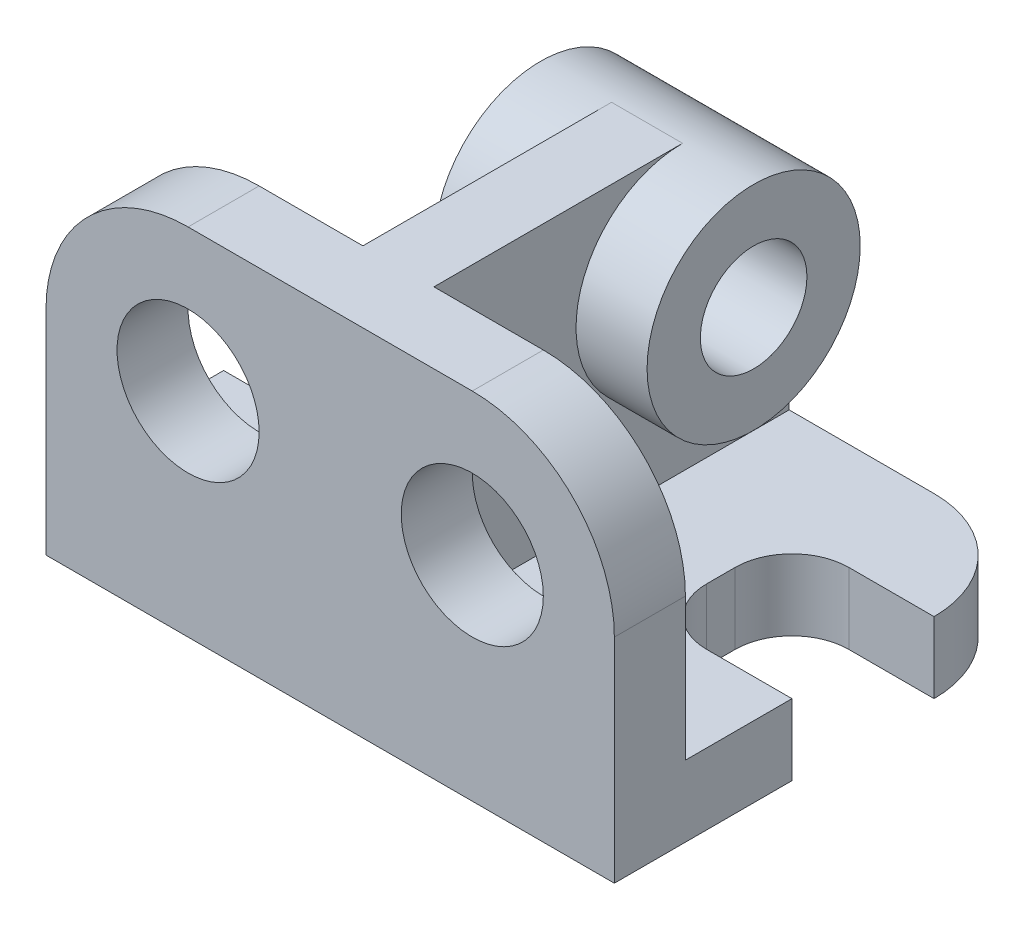
ISO-10303-21;
HEADER;
FILE_DESCRIPTION(('STEP AP214'),'2;1');
FILE_NAME('part.step','',(''),(''),'','','');
FILE_SCHEMA(('AUTOMOTIVE_DESIGN { 1 0 10303 214 1 1 1 1 }'));
ENDSEC;
DATA;
#1=APPLICATION_CONTEXT('core data for automotive mechanical design processes');
#2=APPLICATION_PROTOCOL_DEFINITION('international standard','automotive_design',2000,#1);
#3=PRODUCT_CONTEXT('',#1,'mechanical');
#4=PRODUCT('Part','Part','',(#3));
#5=PRODUCT_RELATED_PRODUCT_CATEGORY('part','',(#4));
#6=PRODUCT_DEFINITION_FORMATION('','',#4);
#7=PRODUCT_DEFINITION_CONTEXT('part definition',#1,'design');
#8=PRODUCT_DEFINITION('design','',#6,#7);
#9=PRODUCT_DEFINITION_SHAPE('','',#8);
#10=(LENGTH_UNIT() NAMED_UNIT(*) SI_UNIT(.MILLI.,.METRE.));
#11=(NAMED_UNIT(*) PLANE_ANGLE_UNIT() SI_UNIT($,.RADIAN.));
#12=(NAMED_UNIT(*) SI_UNIT($,.STERADIAN.) SOLID_ANGLE_UNIT());
#13=UNCERTAINTY_MEASURE_WITH_UNIT(LENGTH_MEASURE(1.E-05),#10,'distance_accuracy_value','');
#14=(GEOMETRIC_REPRESENTATION_CONTEXT(3) GLOBAL_UNCERTAINTY_ASSIGNED_CONTEXT((#13)) GLOBAL_UNIT_ASSIGNED_CONTEXT((#10,
#11,#12)) REPRESENTATION_CONTEXT('',''));
#15=CARTESIAN_POINT('',(0.,0.,0.));
#16=DIRECTION('',(0.,0.,1.));
#17=DIRECTION('',(1.,0.,0.));
#18=AXIS2_PLACEMENT_3D('',#15,#16,#17);
#19=CARTESIAN_POINT('',(-2.49999999999999,1.,-3.));
#20=DIRECTION('',(0.,0.,1.));
#21=DIRECTION('',(1.,0.,0.));
#22=AXIS2_PLACEMENT_3D('',#19,#20,#21);
#23=PLANE('',#22);
#24=DIRECTION('',(1.,0.,0.));
#25=VECTOR('',#24,1.);
#26=CARTESIAN_POINT('',(-2.53950180731732,3.5,-3.));
#27=LINE('',#26,#25);
#28=CARTESIAN_POINT('',(-0.539501807317321,3.5,-3.));
#29=VERTEX_POINT('',#28);
#30=CARTESIAN_POINT('',(0.460498192682678,3.5,-3.));
#31=VERTEX_POINT('',#30);
#32=EDGE_CURVE('E202',#29,#31,#27,.T.);
#33=ORIENTED_EDGE('',*,*,#32,.T.);
#34=DIRECTION('',(0.,-1.,0.));
#35=VECTOR('',#34,1.);
#36=CARTESIAN_POINT('',(0.460498192682678,1.,-3.));
#37=LINE('',#36,#35);
#38=CARTESIAN_POINT('',(0.460498192682678,1.,-3.));
#39=VERTEX_POINT('',#38);
#40=EDGE_CURVE('E208',#31,#39,#37,.T.);
#41=ORIENTED_EDGE('',*,*,#40,.T.);
#42=DIRECTION('',(-1.,0.,0.));
#43=VECTOR('',#42,1.);
#44=CARTESIAN_POINT('',(-2.49999999999999,1.,-3.));
#45=LINE('',#44,#43);
#46=CARTESIAN_POINT('',(2.49999999999999,1.,-3.));
#47=VERTEX_POINT('',#46);
#48=EDGE_CURVE('E307',#47,#39,#45,.T.);
#49=ORIENTED_EDGE('',*,*,#48,.F.);
#50=DIRECTION('',(0.,-1.,0.));
#51=VECTOR('',#50,1.);
#52=CARTESIAN_POINT('',(2.49999999999999,1.,-3.));
#53=LINE('',#52,#51);
#54=CARTESIAN_POINT('',(2.49999999999999,0.,-3.));
#55=VERTEX_POINT('',#54);
#56=EDGE_CURVE('E375',#47,#55,#53,.T.);
#57=ORIENTED_EDGE('',*,*,#56,.T.);
#58=DIRECTION('',(-1.,0.,0.));
#59=VECTOR('',#58,1.);
#60=CARTESIAN_POINT('',(-2.49999999999999,0.,-3.));
#61=LINE('',#60,#59);
#62=CARTESIAN_POINT('',(-2.49999999999999,0.,-3.));
#63=VERTEX_POINT('',#62);
#64=EDGE_CURVE('E338',#55,#63,#61,.T.);
#65=ORIENTED_EDGE('',*,*,#64,.T.);
#66=DIRECTION('',(0.,-1.,0.));
#67=VECTOR('',#66,1.);
#68=CARTESIAN_POINT('',(-2.49999999999999,1.,-3.));
#69=LINE('',#68,#67);
#70=CARTESIAN_POINT('',(-2.49999999999999,1.,-3.));
#71=VERTEX_POINT('',#70);
#72=EDGE_CURVE('E369',#71,#63,#69,.T.);
#73=ORIENTED_EDGE('',*,*,#72,.F.);
#74=CARTESIAN_POINT('',(-0.539501807317322,1.,-3.));
#75=VERTEX_POINT('',#74);
#76=EDGE_CURVE('E308',#75,#71,#45,.T.);
#77=ORIENTED_EDGE('',*,*,#76,.F.);
#78=DIRECTION('',(0.,1.,0.));
#79=VECTOR('',#78,1.);
#80=CARTESIAN_POINT('',(-0.539501807317321,5.,-3.));
#81=LINE('',#80,#79);
#82=EDGE_CURVE('E211',#75,#29,#81,.T.);
#83=ORIENTED_EDGE('',*,*,#82,.T.);
#84=EDGE_LOOP('',(#33,#41,#49,#57,#65,#73,#77,#83));
#85=FACE_BOUND('',#84,.T.);
#86=ADVANCED_FACE('F39',(#85),#23,.F.);
#87=CARTESIAN_POINT('',(-1.99999999999999,5.,2.));
#88=DIRECTION('',(0.,1.,0.));
#89=DIRECTION('',(0.,0.,1.));
#90=AXIS2_PLACEMENT_3D('',#87,#88,#89);
#91=PLANE('',#90);
#92=DIRECTION('',(0.,0.,1.));
#93=VECTOR('',#92,1.);
#94=CARTESIAN_POINT('',(0.460498192682678,5.,-3.));
#95=LINE('',#94,#93);
#96=CARTESIAN_POINT('',(0.460498192682678,5.,-1.5));
#97=VERTEX_POINT('',#96);
#98=CARTESIAN_POINT('',(0.460498192682678,5.,2.));
#99=VERTEX_POINT('',#98);
#100=EDGE_CURVE('E233',#97,#99,#95,.T.);
#101=ORIENTED_EDGE('',*,*,#100,.F.);
#102=DIRECTION('',(1.,0.,0.));
#103=VECTOR('',#102,1.);
#104=CARTESIAN_POINT('',(-2.53950180731732,5.,-1.5));
#105=LINE('',#104,#103);
#106=CARTESIAN_POINT('',(-0.539501807317321,5.,-1.5));
#107=VERTEX_POINT('',#106);
#108=EDGE_CURVE('E53',#107,#97,#105,.T.);
#109=ORIENTED_EDGE('',*,*,#108,.F.);
#110=DIRECTION('',(0.,0.,1.));
#111=VECTOR('',#110,1.);
#112=CARTESIAN_POINT('',(-0.539501807317321,5.,-3.));
#113=LINE('',#112,#111);
#114=CARTESIAN_POINT('',(-0.539501807317322,5.,2.));
#115=VERTEX_POINT('',#114);
#116=EDGE_CURVE('E58',#107,#115,#113,.T.);
#117=ORIENTED_EDGE('',*,*,#116,.T.);
#118=DIRECTION('',(-1.,0.,0.));
#119=VECTOR('',#118,1.);
#120=CARTESIAN_POINT('',(-1.99999999999999,5.,2.));
#121=LINE('',#120,#119);
#122=CARTESIAN_POINT('',(-1.99999999999999,5.,2.));
#123=VERTEX_POINT('',#122);
#124=EDGE_CURVE('E265',#115,#123,#121,.T.);
#125=ORIENTED_EDGE('',*,*,#124,.T.);
#126=DIRECTION('',(0.,0.,1.));
#127=VECTOR('',#126,1.);
#128=CARTESIAN_POINT('',(-1.99999999999999,5.,2.));
#129=LINE('',#128,#127);
#130=CARTESIAN_POINT('',(-1.99999999999999,5.,3.));
#131=VERTEX_POINT('',#130);
#132=EDGE_CURVE('E273',#123,#131,#129,.T.);
#133=ORIENTED_EDGE('',*,*,#132,.T.);
#134=DIRECTION('',(-1.,0.,0.));
#135=VECTOR('',#134,1.);
#136=CARTESIAN_POINT('',(-1.99999999999999,5.,3.));
#137=LINE('',#136,#135);
#138=CARTESIAN_POINT('',(1.99999999999999,5.,3.));
#139=VERTEX_POINT('',#138);
#140=EDGE_CURVE('E255',#139,#131,#137,.T.);
#141=ORIENTED_EDGE('',*,*,#140,.F.);
#142=DIRECTION('',(0.,0.,1.));
#143=VECTOR('',#142,1.);
#144=CARTESIAN_POINT('',(1.99999999999999,5.,2.));
#145=LINE('',#144,#143);
#146=CARTESIAN_POINT('',(1.99999999999999,5.,2.));
#147=VERTEX_POINT('',#146);
#148=EDGE_CURVE('E280',#147,#139,#145,.T.);
#149=ORIENTED_EDGE('',*,*,#148,.F.);
#150=EDGE_CURVE('E263',#147,#99,#121,.T.);
#151=ORIENTED_EDGE('',*,*,#150,.T.);
#152=EDGE_LOOP('',(#101,#109,#117,#125,#133,#141,#149,#151));
#153=FACE_BOUND('',#152,.T.);
#154=ADVANCED_FACE('F453',(#153),#91,.T.);
#155=CARTESIAN_POINT('',(-0.539501807317321,5.,-3.));
#156=DIRECTION('',(1.,0.,0.));
#157=DIRECTION('',(0.,1.,0.));
#158=AXIS2_PLACEMENT_3D('',#155,#156,#157);
#159=PLANE('',#158);
#160=ORIENTED_EDGE('',*,*,#116,.F.);
#161=CARTESIAN_POINT('',(-0.539501807317322,3.5,-1.5));
#162=DIRECTION('',(1.,0.,0.));
#163=DIRECTION('',(0.,1.,0.));
#164=AXIS2_PLACEMENT_3D('',#161,#162,#163);
#165=CIRCLE('',#164,1.5);
#166=EDGE_CURVE('E231',#107,#29,#165,.T.);
#167=ORIENTED_EDGE('',*,*,#166,.T.);
#168=ORIENTED_EDGE('',*,*,#82,.F.);
#169=DIRECTION('',(0.,0.,1.));
#170=VECTOR('',#169,1.);
#171=CARTESIAN_POINT('',(-0.539501807317322,1.,-3.));
#172=LINE('',#171,#170);
#173=CARTESIAN_POINT('',(-0.539501807317322,1.,2.));
#174=VERTEX_POINT('',#173);
#175=EDGE_CURVE('E225',#75,#174,#172,.T.);
#176=ORIENTED_EDGE('',*,*,#175,.T.);
#177=DIRECTION('',(0.,1.,0.));
#178=VECTOR('',#177,1.);
#179=CARTESIAN_POINT('',(-0.539501807317321,5.,2.));
#180=LINE('',#179,#178);
#181=EDGE_CURVE('E228',#174,#115,#180,.T.);
#182=ORIENTED_EDGE('',*,*,#181,.T.);
#183=EDGE_LOOP('',(#160,#167,#168,#176,#182));
#184=FACE_BOUND('',#183,.T.);
#185=ADVANCED_FACE('F478',(#184),#159,.F.);
#186=CARTESIAN_POINT('',(-2.8,1.,-0.3));
#187=DIRECTION('',(0.,-1.,0.));
#188=DIRECTION('',(0.,0.,-1.));
#189=AXIS2_PLACEMENT_3D('',#186,#187,#188);
#190=PLANE('',#189);
#191=ORIENTED_EDGE('',*,*,#175,.F.);
#192=ORIENTED_EDGE('',*,*,#76,.T.);
#193=CARTESIAN_POINT('',(-2.5,1.,-1.5));
#194=DIRECTION('',(0.,1.,0.));
#195=DIRECTION('',(0.,0.,1.));
#196=AXIS2_PLACEMENT_3D('',#193,#194,#195);
#197=CIRCLE('',#196,1.5);
#198=CARTESIAN_POINT('',(-4.,1.,-1.49999999999999));
#199=VERTEX_POINT('',#198);
#200=EDGE_CURVE('E310',#71,#199,#197,.T.);
#201=ORIENTED_EDGE('',*,*,#200,.T.);
#202=DIRECTION('',(1.,0.,0.));
#203=VECTOR('',#202,1.);
#204=CARTESIAN_POINT('',(-4.,1.,-1.49999999999999));
#205=LINE('',#204,#203);
#206=CARTESIAN_POINT('',(-2.80000000000001,1.,-1.5));
#207=VERTEX_POINT('',#206);
#208=EDGE_CURVE('E313',#199,#207,#205,.T.);
#209=ORIENTED_EDGE('',*,*,#208,.T.);
#210=CARTESIAN_POINT('',(-2.8,1.,-0.699999999999996));
#211=DIRECTION('',(0.,-1.,0.));
#212=DIRECTION('',(0.,0.,1.));
#213=AXIS2_PLACEMENT_3D('',#210,#211,#212);
#214=CIRCLE('',#213,0.8);
#215=CARTESIAN_POINT('',(-2.,1.,-0.69999999999999));
#216=VERTEX_POINT('',#215);
#217=EDGE_CURVE('E311',#207,#216,#214,.T.);
#218=ORIENTED_EDGE('',*,*,#217,.T.);
#219=DIRECTION('',(0.,0.,1.));
#220=VECTOR('',#219,1.);
#221=CARTESIAN_POINT('',(-2.,1.,-0.69999999999999));
#222=LINE('',#221,#220);
#223=CARTESIAN_POINT('',(-2.,1.,-0.300000000000006));
#224=VERTEX_POINT('',#223);
#225=EDGE_CURVE('E312',#216,#224,#222,.T.);
#226=ORIENTED_EDGE('',*,*,#225,.T.);
#227=CARTESIAN_POINT('',(-2.8,1.,-0.3));
#228=DIRECTION('',(0.,-1.,0.));
#229=DIRECTION('',(0.,0.,-1.));
#230=AXIS2_PLACEMENT_3D('',#227,#228,#229);
#231=CIRCLE('',#230,0.8);
#232=CARTESIAN_POINT('',(-2.80000000000001,1.,0.5));
#233=VERTEX_POINT('',#232);
#234=EDGE_CURVE('E320',#224,#233,#231,.T.);
#235=ORIENTED_EDGE('',*,*,#234,.T.);
#236=DIRECTION('',(-1.,0.,0.));
#237=VECTOR('',#236,1.);
#238=CARTESIAN_POINT('',(-2.80000000000001,1.,0.5));
#239=LINE('',#238,#237);
#240=CARTESIAN_POINT('',(-4.,1.,0.5));
#241=VERTEX_POINT('',#240);
#242=EDGE_CURVE('E317',#233,#241,#239,.T.);
#243=ORIENTED_EDGE('',*,*,#242,.T.);
#244=DIRECTION('',(0.,0.,1.));
#245=VECTOR('',#244,1.);
#246=CARTESIAN_POINT('',(-4.,1.,3.));
#247=LINE('',#246,#245);
#248=CARTESIAN_POINT('',(-4.,1.,2.));
#249=VERTEX_POINT('',#248);
#250=EDGE_CURVE('E289',#241,#249,#247,.T.);
#251=ORIENTED_EDGE('',*,*,#250,.T.);
#252=DIRECTION('',(-1.,0.,0.));
#253=VECTOR('',#252,1.);
#254=CARTESIAN_POINT('',(-2.8,1.,2.));
#255=LINE('',#254,#253);
#256=EDGE_CURVE('E277',#174,#249,#255,.T.);
#257=ORIENTED_EDGE('',*,*,#256,.F.);
#258=EDGE_LOOP('',(#191,#192,#201,#209,#218,#226,#235,#243,#251,#257));
#259=FACE_BOUND('',#258,.T.);
#260=ADVANCED_FACE('F417',(#259),#190,.F.);
#261=DIRECTION('',(0.,0.,1.));
#262=VECTOR('',#261,1.);
#263=CARTESIAN_POINT('',(0.460498192682678,1.,-3.));
#264=LINE('',#263,#262);
#265=CARTESIAN_POINT('',(0.460498192682678,1.,2.));
#266=VERTEX_POINT('',#265);
#267=EDGE_CURVE('E219',#39,#266,#264,.T.);
#268=ORIENTED_EDGE('',*,*,#267,.T.);
#269=CARTESIAN_POINT('',(4.,1.,2.));
#270=VERTEX_POINT('',#269);
#271=EDGE_CURVE('E283',#270,#266,#255,.T.);
#272=ORIENTED_EDGE('',*,*,#271,.F.);
#273=DIRECTION('',(0.,0.,-1.));
#274=VECTOR('',#273,1.);
#275=CARTESIAN_POINT('',(4.,1.,3.));
#276=LINE('',#275,#274);
#277=CARTESIAN_POINT('',(4.,1.,0.5));
#278=VERTEX_POINT('',#277);
#279=EDGE_CURVE('E292',#270,#278,#276,.T.);
#280=ORIENTED_EDGE('',*,*,#279,.T.);
#281=DIRECTION('',(-1.,0.,0.));
#282=VECTOR('',#281,1.);
#283=CARTESIAN_POINT('',(2.80000000000001,1.,0.5));
#284=LINE('',#283,#282);
#285=CARTESIAN_POINT('',(2.80000000000001,1.,0.5));
#286=VERTEX_POINT('',#285);
#287=EDGE_CURVE('E294',#278,#286,#284,.T.);
#288=ORIENTED_EDGE('',*,*,#287,.T.);
#289=CARTESIAN_POINT('',(2.8,1.,-0.3));
#290=DIRECTION('',(0.,-1.,0.));
#291=DIRECTION('',(0.,0.,1.));
#292=AXIS2_PLACEMENT_3D('',#289,#290,#291);
#293=CIRCLE('',#292,0.8);
#294=CARTESIAN_POINT('',(2.,1.,-0.300000000000006));
#295=VERTEX_POINT('',#294);
#296=EDGE_CURVE('E296',#286,#295,#293,.T.);
#297=ORIENTED_EDGE('',*,*,#296,.T.);
#298=DIRECTION('',(0.,0.,-1.));
#299=VECTOR('',#298,1.);
#300=CARTESIAN_POINT('',(2.,1.,-0.69999999999999));
#301=LINE('',#300,#299);
#302=CARTESIAN_POINT('',(2.,1.,-0.69999999999999));
#303=VERTEX_POINT('',#302);
#304=EDGE_CURVE('E299',#295,#303,#301,.T.);
#305=ORIENTED_EDGE('',*,*,#304,.T.);
#306=CARTESIAN_POINT('',(2.8,1.,-0.699999999999996));
#307=DIRECTION('',(0.,-1.,0.));
#308=DIRECTION('',(0.,0.,-1.));
#309=AXIS2_PLACEMENT_3D('',#306,#307,#308);
#310=CIRCLE('',#309,0.8);
#311=CARTESIAN_POINT('',(2.8,1.,-1.5));
#312=VERTEX_POINT('',#311);
#313=EDGE_CURVE('E300',#303,#312,#310,.T.);
#314=ORIENTED_EDGE('',*,*,#313,.T.);
#315=DIRECTION('',(1.,0.,0.));
#316=VECTOR('',#315,1.);
#317=CARTESIAN_POINT('',(4.,1.,-1.49999999999999));
#318=LINE('',#317,#316);
#319=CARTESIAN_POINT('',(4.,1.,-1.49999999999999));
#320=VERTEX_POINT('',#319);
#321=EDGE_CURVE('E302',#312,#320,#318,.T.);
#322=ORIENTED_EDGE('',*,*,#321,.T.);
#323=CARTESIAN_POINT('',(2.5,1.,-1.5));
#324=DIRECTION('',(0.,1.,0.));
#325=DIRECTION('',(0.,0.,-1.));
#326=AXIS2_PLACEMENT_3D('',#323,#324,#325);
#327=CIRCLE('',#326,1.5);
#328=EDGE_CURVE('E303',#320,#47,#327,.T.);
#329=ORIENTED_EDGE('',*,*,#328,.T.);
#330=ORIENTED_EDGE('',*,*,#48,.T.);
#331=EDGE_LOOP('',(#268,#272,#280,#288,#297,#305,#314,#322,#329,#330));
#332=FACE_BOUND('',#331,.T.);
#333=ADVANCED_FACE('F442',(#332),#190,.F.);
#334=CARTESIAN_POINT('',(-2.,3.,2.));
#335=DIRECTION('',(0.,0.,1.));
#336=DIRECTION('',(1.,0.,0.));
#337=AXIS2_PLACEMENT_3D('',#334,#335,#336);
#338=PLANE('',#337);
#339=CARTESIAN_POINT('',(-2.,3.,2.));
#340=DIRECTION('',(0.,0.,1.));
#341=DIRECTION('',(1.,0.,0.));
#342=AXIS2_PLACEMENT_3D('',#339,#340,#341);
#343=CIRCLE('',#342,1.);
#344=CARTESIAN_POINT('',(-1.,3.,2.));
#345=VERTEX_POINT('',#344);
#346=EDGE_CURVE('E243',#345,#345,#343,.T.);
#347=ORIENTED_EDGE('',*,*,#346,.T.);
#348=EDGE_LOOP('',(#347));
#349=FACE_BOUND('',#348,.T.);
#350=ORIENTED_EDGE('',*,*,#181,.F.);
#351=ORIENTED_EDGE('',*,*,#256,.T.);
#352=DIRECTION('',(0.,-1.,0.));
#353=VECTOR('',#352,1.);
#354=CARTESIAN_POINT('',(-4.,0.,2.));
#355=LINE('',#354,#353);
#356=CARTESIAN_POINT('',(-4.,2.99999999999999,2.));
#357=VERTEX_POINT('',#356);
#358=EDGE_CURVE('E251',#357,#249,#355,.T.);
#359=ORIENTED_EDGE('',*,*,#358,.F.);
#360=CARTESIAN_POINT('',(-2.,3.,2.));
#361=DIRECTION('',(0.,0.,1.));
#362=DIRECTION('',(1.,0.,0.));
#363=AXIS2_PLACEMENT_3D('',#360,#361,#362);
#364=CIRCLE('',#363,2.);
#365=EDGE_CURVE('E250',#123,#357,#364,.T.);
#366=ORIENTED_EDGE('',*,*,#365,.F.);
#367=ORIENTED_EDGE('',*,*,#124,.F.);
#368=EDGE_LOOP('',(#350,#351,#359,#366,#367));
#369=FACE_BOUND('',#368,.T.);
#370=ADVANCED_FACE('F411',(#349,#369),#338,.F.);
#371=CARTESIAN_POINT('',(2.,3.,2.));
#372=DIRECTION('',(0.,0.,1.));
#373=DIRECTION('',(1.,0.,0.));
#374=AXIS2_PLACEMENT_3D('',#371,#372,#373);
#375=CIRCLE('',#374,1.);
#376=CARTESIAN_POINT('',(3.,3.,2.));
#377=VERTEX_POINT('',#376);
#378=EDGE_CURVE('E236',#377,#377,#375,.T.);
#379=ORIENTED_EDGE('',*,*,#378,.T.);
#380=EDGE_LOOP('',(#379));
#381=FACE_BOUND('',#380,.T.);
#382=DIRECTION('',(0.,-1.,0.));
#383=VECTOR('',#382,1.);
#384=CARTESIAN_POINT('',(0.460498192682678,1.,2.));
#385=LINE('',#384,#383);
#386=EDGE_CURVE('E223',#99,#266,#385,.T.);
#387=ORIENTED_EDGE('',*,*,#386,.F.);
#388=ORIENTED_EDGE('',*,*,#150,.F.);
#389=CARTESIAN_POINT('',(2.,3.,2.));
#390=DIRECTION('',(0.,0.,1.));
#391=DIRECTION('',(-1.,0.,0.));
#392=AXIS2_PLACEMENT_3D('',#389,#390,#391);
#393=CIRCLE('',#392,2.);
#394=CARTESIAN_POINT('',(4.,2.99999999999999,2.));
#395=VERTEX_POINT('',#394);
#396=EDGE_CURVE('E259',#395,#147,#393,.T.);
#397=ORIENTED_EDGE('',*,*,#396,.F.);
#398=DIRECTION('',(0.,1.,0.));
#399=VECTOR('',#398,1.);
#400=CARTESIAN_POINT('',(4.,0.,2.));
#401=LINE('',#400,#399);
#402=EDGE_CURVE('E260',#270,#395,#401,.T.);
#403=ORIENTED_EDGE('',*,*,#402,.F.);
#404=ORIENTED_EDGE('',*,*,#271,.T.);
#405=EDGE_LOOP('',(#387,#388,#397,#403,#404));
#406=FACE_BOUND('',#405,.T.);
#407=ADVANCED_FACE('F449',(#381,#406),#338,.F.);
#408=CARTESIAN_POINT('',(-4.,1.,3.));
#409=DIRECTION('',(1.,0.,0.));
#410=DIRECTION('',(0.,0.,-1.));
#411=AXIS2_PLACEMENT_3D('',#408,#409,#410);
#412=PLANE('',#411);
#413=DIRECTION('',(0.,-1.,0.));
#414=VECTOR('',#413,1.);
#415=CARTESIAN_POINT('',(-4.,1.,3.));
#416=LINE('',#415,#414);
#417=CARTESIAN_POINT('',(-4.,2.99999999999999,3.));
#418=VERTEX_POINT('',#417);
#419=CARTESIAN_POINT('',(-4.,0.,3.));
#420=VERTEX_POINT('',#419);
#421=EDGE_CURVE('E50',#418,#420,#416,.T.);
#422=ORIENTED_EDGE('',*,*,#421,.F.);
#423=DIRECTION('',(0.,0.,1.));
#424=VECTOR('',#423,1.);
#425=CARTESIAN_POINT('',(-4.,2.99999999999999,2.));
#426=LINE('',#425,#424);
#427=EDGE_CURVE('E266',#357,#418,#426,.T.);
#428=ORIENTED_EDGE('',*,*,#427,.F.);
#429=ORIENTED_EDGE('',*,*,#358,.T.);
#430=ORIENTED_EDGE('',*,*,#250,.F.);
#431=DIRECTION('',(0.,-1.,0.));
#432=VECTOR('',#431,1.);
#433=CARTESIAN_POINT('',(-4.,1.,0.5));
#434=LINE('',#433,#432);
#435=CARTESIAN_POINT('',(-4.,0.,0.5));
#436=VERTEX_POINT('',#435);
#437=EDGE_CURVE('E321',#241,#436,#434,.T.);
#438=ORIENTED_EDGE('',*,*,#437,.T.);
#439=DIRECTION('',(0.,0.,1.));
#440=VECTOR('',#439,1.);
#441=CARTESIAN_POINT('',(-4.,0.,3.));
#442=LINE('',#441,#440);
#443=EDGE_CURVE('E287',#436,#420,#442,.T.);
#444=ORIENTED_EDGE('',*,*,#443,.T.);
#445=EDGE_LOOP('',(#422,#428,#429,#430,#438,#444));
#446=FACE_BOUND('',#445,.T.);
#447=ADVANCED_FACE('F41',(#446),#412,.F.);
#448=CARTESIAN_POINT('',(-4.,1.,3.));
#449=DIRECTION('',(0.,0.,-1.));
#450=DIRECTION('',(-1.,0.,0.));
#451=AXIS2_PLACEMENT_3D('',#448,#449,#450);
#452=PLANE('',#451);
#453=DIRECTION('',(1.,0.,0.));
#454=VECTOR('',#453,1.);
#455=CARTESIAN_POINT('',(-4.,0.,3.));
#456=LINE('',#455,#454);
#457=CARTESIAN_POINT('',(4.,0.,3.));
#458=VERTEX_POINT('',#457);
#459=EDGE_CURVE('E323',#420,#458,#456,.T.);
#460=ORIENTED_EDGE('',*,*,#459,.T.);
#461=DIRECTION('',(0.,-1.,0.));
#462=VECTOR('',#461,1.);
#463=CARTESIAN_POINT('',(4.,1.,3.));
#464=LINE('',#463,#462);
#465=CARTESIAN_POINT('',(4.,2.99999999999999,3.));
#466=VERTEX_POINT('',#465);
#467=EDGE_CURVE('E394',#466,#458,#464,.T.);
#468=ORIENTED_EDGE('',*,*,#467,.F.);
#469=CARTESIAN_POINT('',(2.,3.,3.));
#470=DIRECTION('',(0.,0.,1.));
#471=DIRECTION('',(-1.,0.,0.));
#472=AXIS2_PLACEMENT_3D('',#469,#470,#471);
#473=CIRCLE('',#472,2.);
#474=EDGE_CURVE('E267',#466,#139,#473,.T.);
#475=ORIENTED_EDGE('',*,*,#474,.T.);
#476=ORIENTED_EDGE('',*,*,#140,.T.);
#477=CARTESIAN_POINT('',(-2.,3.,3.));
#478=DIRECTION('',(0.,0.,1.));
#479=DIRECTION('',(1.,0.,0.));
#480=AXIS2_PLACEMENT_3D('',#477,#478,#479);
#481=CIRCLE('',#480,2.);
#482=EDGE_CURVE('E247',#131,#418,#481,.T.);
#483=ORIENTED_EDGE('',*,*,#482,.T.);
#484=ORIENTED_EDGE('',*,*,#421,.T.);
#485=EDGE_LOOP('',(#460,#468,#475,#476,#483,#484));
#486=FACE_BOUND('',#485,.T.);
#487=CARTESIAN_POINT('',(-2.,3.,3.));
#488=DIRECTION('',(0.,0.,1.));
#489=DIRECTION('',(1.,0.,0.));
#490=AXIS2_PLACEMENT_3D('',#487,#488,#489);
#491=CIRCLE('',#490,1.);
#492=CARTESIAN_POINT('',(-1.,3.,3.));
#493=VERTEX_POINT('',#492);
#494=EDGE_CURVE('E241',#493,#493,#491,.T.);
#495=ORIENTED_EDGE('',*,*,#494,.F.);
#496=EDGE_LOOP('',(#495));
#497=FACE_BOUND('',#496,.T.);
#498=CARTESIAN_POINT('',(2.,3.,3.));
#499=DIRECTION('',(0.,0.,1.));
#500=DIRECTION('',(1.,0.,0.));
#501=AXIS2_PLACEMENT_3D('',#498,#499,#500);
#502=CIRCLE('',#501,1.);
#503=CARTESIAN_POINT('',(3.,3.,3.));
#504=VERTEX_POINT('',#503);
#505=EDGE_CURVE('E240',#504,#504,#502,.T.);
#506=ORIENTED_EDGE('',*,*,#505,.F.);
#507=EDGE_LOOP('',(#506));
#508=FACE_BOUND('',#507,.T.);
#509=ADVANCED_FACE('F397',(#486,#497,#508),#452,.F.);
#510=CARTESIAN_POINT('',(4.,1.,3.));
#511=DIRECTION('',(-1.,0.,0.));
#512=DIRECTION('',(0.,0.,1.));
#513=AXIS2_PLACEMENT_3D('',#510,#511,#512);
#514=PLANE('',#513);
#515=DIRECTION('',(0.,0.,-1.));
#516=VECTOR('',#515,1.);
#517=CARTESIAN_POINT('',(4.,0.,3.));
#518=LINE('',#517,#516);
#519=CARTESIAN_POINT('',(4.,0.,0.5));
#520=VERTEX_POINT('',#519);
#521=EDGE_CURVE('E324',#458,#520,#518,.T.);
#522=ORIENTED_EDGE('',*,*,#521,.T.);
#523=DIRECTION('',(0.,-1.,0.));
#524=VECTOR('',#523,1.);
#525=CARTESIAN_POINT('',(4.,1.,0.5));
#526=LINE('',#525,#524);
#527=EDGE_CURVE('E388',#278,#520,#526,.T.);
#528=ORIENTED_EDGE('',*,*,#527,.F.);
#529=ORIENTED_EDGE('',*,*,#279,.F.);
#530=ORIENTED_EDGE('',*,*,#402,.T.);
#531=DIRECTION('',(0.,0.,1.));
#532=VECTOR('',#531,1.);
#533=CARTESIAN_POINT('',(4.,2.99999999999999,2.));
#534=LINE('',#533,#532);
#535=EDGE_CURVE('E276',#395,#466,#534,.T.);
#536=ORIENTED_EDGE('',*,*,#535,.T.);
#537=ORIENTED_EDGE('',*,*,#467,.T.);
#538=EDGE_LOOP('',(#522,#528,#529,#530,#536,#537));
#539=FACE_BOUND('',#538,.T.);
#540=ADVANCED_FACE('F433',(#539),#514,.F.);
#541=CARTESIAN_POINT('',(2.80000000000001,1.,0.5));
#542=DIRECTION('',(0.,0.,1.));
#543=DIRECTION('',(1.,0.,0.));
#544=AXIS2_PLACEMENT_3D('',#541,#542,#543);
#545=PLANE('',#544);
#546=DIRECTION('',(-1.,0.,0.));
#547=VECTOR('',#546,1.);
#548=CARTESIAN_POINT('',(2.80000000000001,0.,0.5));
#549=LINE('',#548,#547);
#550=CARTESIAN_POINT('',(2.80000000000001,0.,0.5));
#551=VERTEX_POINT('',#550);
#552=EDGE_CURVE('E330',#520,#551,#549,.T.);
#553=ORIENTED_EDGE('',*,*,#552,.T.);
#554=DIRECTION('',(0.,-1.,0.));
#555=VECTOR('',#554,1.);
#556=CARTESIAN_POINT('',(2.80000000000001,1.,0.5));
#557=LINE('',#556,#555);
#558=EDGE_CURVE('E390',#286,#551,#557,.T.);
#559=ORIENTED_EDGE('',*,*,#558,.F.);
#560=ORIENTED_EDGE('',*,*,#287,.F.);
#561=ORIENTED_EDGE('',*,*,#527,.T.);
#562=EDGE_LOOP('',(#553,#559,#560,#561));
#563=FACE_BOUND('',#562,.T.);
#564=ADVANCED_FACE('F440',(#563),#545,.F.);
#565=CARTESIAN_POINT('',(2.8,1.,-0.3));
#566=DIRECTION('',(0.,-1.,0.));
#567=DIRECTION('',(0.,0.,-1.));
#568=AXIS2_PLACEMENT_3D('',#565,#566,#567);
#569=CYLINDRICAL_SURFACE('',#568,0.8);
#570=CARTESIAN_POINT('',(2.8,0.,-0.3));
#571=DIRECTION('',(0.,-1.,0.));
#572=DIRECTION('',(0.,0.,1.));
#573=AXIS2_PLACEMENT_3D('',#570,#571,#572);
#574=CIRCLE('',#573,0.8);
#575=CARTESIAN_POINT('',(2.,0.,-0.300000000000006));
#576=VERTEX_POINT('',#575);
#577=EDGE_CURVE('E328',#551,#576,#574,.T.);
#578=ORIENTED_EDGE('',*,*,#577,.T.);
#579=DIRECTION('',(0.,-1.,0.));
#580=VECTOR('',#579,1.);
#581=CARTESIAN_POINT('',(2.,1.,-0.300000000000006));
#582=LINE('',#581,#580);
#583=EDGE_CURVE('E383',#295,#576,#582,.T.);
#584=ORIENTED_EDGE('',*,*,#583,.F.);
#585=ORIENTED_EDGE('',*,*,#296,.F.);
#586=ORIENTED_EDGE('',*,*,#558,.T.);
#587=EDGE_LOOP('',(#578,#584,#585,#586));
#588=FACE_BOUND('',#587,.T.);
#589=ADVANCED_FACE('F538',(#588),#569,.F.);
#590=CARTESIAN_POINT('',(2.,1.,-0.69999999999999));
#591=DIRECTION('',(-1.,0.,0.));
#592=DIRECTION('',(0.,0.,1.));
#593=AXIS2_PLACEMENT_3D('',#590,#591,#592);
#594=PLANE('',#593);
#595=DIRECTION('',(0.,0.,-1.));
#596=VECTOR('',#595,1.);
#597=CARTESIAN_POINT('',(2.,0.,-0.69999999999999));
#598=LINE('',#597,#596);
#599=CARTESIAN_POINT('',(2.,0.,-0.69999999999999));
#600=VERTEX_POINT('',#599);
#601=EDGE_CURVE('E332',#576,#600,#598,.T.);
#602=ORIENTED_EDGE('',*,*,#601,.T.);
#603=DIRECTION('',(0.,-1.,0.));
#604=VECTOR('',#603,1.);
#605=CARTESIAN_POINT('',(2.,1.,-0.69999999999999));
#606=LINE('',#605,#604);
#607=EDGE_CURVE('E381',#303,#600,#606,.T.);
#608=ORIENTED_EDGE('',*,*,#607,.F.);
#609=ORIENTED_EDGE('',*,*,#304,.F.);
#610=ORIENTED_EDGE('',*,*,#583,.T.);
#611=EDGE_LOOP('',(#602,#608,#609,#610));
#612=FACE_BOUND('',#611,.T.);
#613=ADVANCED_FACE('F534',(#612),#594,.F.);
#614=CARTESIAN_POINT('',(2.8,1.,-0.699999999999996));
#615=DIRECTION('',(0.,-1.,0.));
#616=DIRECTION('',(0.,0.,-1.));
#617=AXIS2_PLACEMENT_3D('',#614,#615,#616);
#618=CYLINDRICAL_SURFACE('',#617,0.8);
#619=CARTESIAN_POINT('',(2.8,0.,-0.699999999999996));
#620=DIRECTION('',(0.,-1.,0.));
#621=DIRECTION('',(0.,0.,-1.));
#622=AXIS2_PLACEMENT_3D('',#619,#620,#621);
#623=CIRCLE('',#622,0.8);
#624=CARTESIAN_POINT('',(2.8,0.,-1.5));
#625=VERTEX_POINT('',#624);
#626=EDGE_CURVE('E334',#600,#625,#623,.T.);
#627=ORIENTED_EDGE('',*,*,#626,.T.);
#628=DIRECTION('',(0.,-1.,0.));
#629=VECTOR('',#628,1.);
#630=CARTESIAN_POINT('',(2.8,1.,-1.5));
#631=LINE('',#630,#629);
#632=EDGE_CURVE('E378',#312,#625,#631,.T.);
#633=ORIENTED_EDGE('',*,*,#632,.F.);
#634=ORIENTED_EDGE('',*,*,#313,.F.);
#635=ORIENTED_EDGE('',*,*,#607,.T.);
#636=EDGE_LOOP('',(#627,#633,#634,#635));
#637=FACE_BOUND('',#636,.T.);
#638=ADVANCED_FACE('F529',(#637),#618,.F.);
#639=CARTESIAN_POINT('',(4.,1.,-1.49999999999999));
#640=DIRECTION('',(0.,0.,-1.));
#641=DIRECTION('',(-1.,0.,0.));
#642=AXIS2_PLACEMENT_3D('',#639,#640,#641);
#643=PLANE('',#642);
#644=DIRECTION('',(1.,0.,0.));
#645=VECTOR('',#644,1.);
#646=CARTESIAN_POINT('',(4.,0.,-1.49999999999999));
#647=LINE('',#646,#645);
#648=CARTESIAN_POINT('',(4.,0.,-1.49999999999999));
#649=VERTEX_POINT('',#648);
#650=EDGE_CURVE('E333',#625,#649,#647,.T.);
#651=ORIENTED_EDGE('',*,*,#650,.T.);
#652=DIRECTION('',(0.,-1.,0.));
#653=VECTOR('',#652,1.);
#654=CARTESIAN_POINT('',(4.,1.,-1.49999999999999));
#655=LINE('',#654,#653);
#656=EDGE_CURVE('E374',#320,#649,#655,.T.);
#657=ORIENTED_EDGE('',*,*,#656,.F.);
#658=ORIENTED_EDGE('',*,*,#321,.F.);
#659=ORIENTED_EDGE('',*,*,#632,.T.);
#660=EDGE_LOOP('',(#651,#657,#658,#659));
#661=FACE_BOUND('',#660,.T.);
#662=ADVANCED_FACE('F527',(#661),#643,.F.);
#663=CARTESIAN_POINT('',(2.5,1.,-1.5));
#664=DIRECTION('',(0.,-1.,0.));
#665=DIRECTION('',(0.,0.,-1.));
#666=AXIS2_PLACEMENT_3D('',#663,#664,#665);
#667=CYLINDRICAL_SURFACE('',#666,1.5);
#668=CARTESIAN_POINT('',(2.5,0.,-1.5));
#669=DIRECTION('',(0.,1.,0.));
#670=DIRECTION('',(0.,0.,-1.));
#671=AXIS2_PLACEMENT_3D('',#668,#669,#670);
#672=CIRCLE('',#671,1.5);
#673=EDGE_CURVE('E337',#649,#55,#672,.T.);
#674=ORIENTED_EDGE('',*,*,#673,.T.);
#675=ORIENTED_EDGE('',*,*,#56,.F.);
#676=ORIENTED_EDGE('',*,*,#328,.F.);
#677=ORIENTED_EDGE('',*,*,#656,.T.);
#678=EDGE_LOOP('',(#674,#675,#676,#677));
#679=FACE_BOUND('',#678,.T.);
#680=ADVANCED_FACE('F523',(#679),#667,.T.);
#681=CARTESIAN_POINT('',(-2.5,1.,-1.5));
#682=DIRECTION('',(0.,-1.,0.));
#683=DIRECTION('',(0.,0.,-1.));
#684=AXIS2_PLACEMENT_3D('',#681,#682,#683);
#685=CYLINDRICAL_SURFACE('',#684,1.5);
#686=CARTESIAN_POINT('',(-2.5,0.,-1.5));
#687=DIRECTION('',(0.,1.,0.));
#688=DIRECTION('',(0.,0.,1.));
#689=AXIS2_PLACEMENT_3D('',#686,#687,#688);
#690=CIRCLE('',#689,1.5);
#691=CARTESIAN_POINT('',(-4.,0.,-1.49999999999999));
#692=VERTEX_POINT('',#691);
#693=EDGE_CURVE('E341',#63,#692,#690,.T.);
#694=ORIENTED_EDGE('',*,*,#693,.T.);
#695=DIRECTION('',(0.,-1.,0.));
#696=VECTOR('',#695,1.);
#697=CARTESIAN_POINT('',(-4.,1.,-1.49999999999999));
#698=LINE('',#697,#696);
#699=EDGE_CURVE('E368',#199,#692,#698,.T.);
#700=ORIENTED_EDGE('',*,*,#699,.F.);
#701=ORIENTED_EDGE('',*,*,#200,.F.);
#702=ORIENTED_EDGE('',*,*,#72,.T.);
#703=EDGE_LOOP('',(#694,#700,#701,#702));
#704=FACE_BOUND('',#703,.T.);
#705=ADVANCED_FACE('F467',(#704),#685,.T.);
#706=CARTESIAN_POINT('',(-4.,1.,-1.49999999999999));
#707=DIRECTION('',(0.,0.,-1.));
#708=DIRECTION('',(-1.,0.,0.));
#709=AXIS2_PLACEMENT_3D('',#706,#707,#708);
#710=PLANE('',#709);
#711=DIRECTION('',(1.,0.,0.));
#712=VECTOR('',#711,1.);
#713=CARTESIAN_POINT('',(-4.,0.,-1.49999999999999));
#714=LINE('',#713,#712);
#715=CARTESIAN_POINT('',(-2.80000000000001,0.,-1.5));
#716=VERTEX_POINT('',#715);
#717=EDGE_CURVE('E344',#692,#716,#714,.T.);
#718=ORIENTED_EDGE('',*,*,#717,.T.);
#719=DIRECTION('',(0.,-1.,0.));
#720=VECTOR('',#719,1.);
#721=CARTESIAN_POINT('',(-2.80000000000001,1.,-1.5));
#722=LINE('',#721,#720);
#723=EDGE_CURVE('E361',#207,#716,#722,.T.);
#724=ORIENTED_EDGE('',*,*,#723,.F.);
#725=ORIENTED_EDGE('',*,*,#208,.F.);
#726=ORIENTED_EDGE('',*,*,#699,.T.);
#727=EDGE_LOOP('',(#718,#724,#725,#726));
#728=FACE_BOUND('',#727,.T.);
#729=ADVANCED_FACE('F473',(#728),#710,.F.);
#730=CARTESIAN_POINT('',(-2.8,1.,-0.699999999999996));
#731=DIRECTION('',(0.,-1.,0.));
#732=DIRECTION('',(0.,0.,-1.));
#733=AXIS2_PLACEMENT_3D('',#730,#731,#732);
#734=CYLINDRICAL_SURFACE('',#733,0.8);
#735=CARTESIAN_POINT('',(-2.8,0.,-0.699999999999996));
#736=DIRECTION('',(0.,-1.,0.));
#737=DIRECTION('',(0.,0.,1.));
#738=AXIS2_PLACEMENT_3D('',#735,#736,#737);
#739=CIRCLE('',#738,0.8);
#740=CARTESIAN_POINT('',(-2.,0.,-0.69999999999999));
#741=VERTEX_POINT('',#740);
#742=EDGE_CURVE('E345',#716,#741,#739,.T.);
#743=ORIENTED_EDGE('',*,*,#742,.T.);
#744=DIRECTION('',(0.,-1.,0.));
#745=VECTOR('',#744,1.);
#746=CARTESIAN_POINT('',(-2.,1.,-0.69999999999999));
#747=LINE('',#746,#745);
#748=EDGE_CURVE('E360',#216,#741,#747,.T.);
#749=ORIENTED_EDGE('',*,*,#748,.F.);
#750=ORIENTED_EDGE('',*,*,#217,.F.);
#751=ORIENTED_EDGE('',*,*,#723,.T.);
#752=EDGE_LOOP('',(#743,#749,#750,#751));
#753=FACE_BOUND('',#752,.T.);
#754=ADVANCED_FACE('F580',(#753),#734,.F.);
#755=CARTESIAN_POINT('',(-2.,1.,-0.69999999999999));
#756=DIRECTION('',(1.,0.,0.));
#757=DIRECTION('',(0.,0.,-1.));
#758=AXIS2_PLACEMENT_3D('',#755,#756,#757);
#759=PLANE('',#758);
#760=DIRECTION('',(0.,0.,1.));
#761=VECTOR('',#760,1.);
#762=CARTESIAN_POINT('',(-2.,0.,-0.69999999999999));
#763=LINE('',#762,#761);
#764=CARTESIAN_POINT('',(-2.,0.,-0.300000000000006));
#765=VERTEX_POINT('',#764);
#766=EDGE_CURVE('E350',#741,#765,#763,.T.);
#767=ORIENTED_EDGE('',*,*,#766,.T.);
#768=DIRECTION('',(0.,-1.,0.));
#769=VECTOR('',#768,1.);
#770=CARTESIAN_POINT('',(-2.,1.,-0.300000000000006));
#771=LINE('',#770,#769);
#772=EDGE_CURVE('E357',#224,#765,#771,.T.);
#773=ORIENTED_EDGE('',*,*,#772,.F.);
#774=ORIENTED_EDGE('',*,*,#225,.F.);
#775=ORIENTED_EDGE('',*,*,#748,.T.);
#776=EDGE_LOOP('',(#767,#773,#774,#775));
#777=FACE_BOUND('',#776,.T.);
#778=ADVANCED_FACE('F576',(#777),#759,.F.);
#779=CARTESIAN_POINT('',(-2.8,1.,-0.3));
#780=DIRECTION('',(0.,-1.,0.));
#781=DIRECTION('',(0.,0.,-1.));
#782=AXIS2_PLACEMENT_3D('',#779,#780,#781);
#783=CYLINDRICAL_SURFACE('',#782,0.8);
#784=CARTESIAN_POINT('',(-2.8,0.,-0.3));
#785=DIRECTION('',(0.,-1.,0.));
#786=DIRECTION('',(0.,0.,-1.));
#787=AXIS2_PLACEMENT_3D('',#784,#785,#786);
#788=CIRCLE('',#787,0.8);
#789=CARTESIAN_POINT('',(-2.80000000000001,0.,0.5));
#790=VERTEX_POINT('',#789);
#791=EDGE_CURVE('E349',#765,#790,#788,.T.);
#792=ORIENTED_EDGE('',*,*,#791,.T.);
#793=DIRECTION('',(0.,-1.,0.));
#794=VECTOR('',#793,1.);
#795=CARTESIAN_POINT('',(-2.80000000000001,1.,0.5));
#796=LINE('',#795,#794);
#797=EDGE_CURVE('E353',#233,#790,#796,.T.);
#798=ORIENTED_EDGE('',*,*,#797,.F.);
#799=ORIENTED_EDGE('',*,*,#234,.F.);
#800=ORIENTED_EDGE('',*,*,#772,.T.);
#801=EDGE_LOOP('',(#792,#798,#799,#800));
#802=FACE_BOUND('',#801,.T.);
#803=ADVANCED_FACE('F574',(#802),#783,.F.);
#804=CARTESIAN_POINT('',(-2.80000000000001,1.,0.5));
#805=DIRECTION('',(0.,0.,1.));
#806=DIRECTION('',(1.,0.,0.));
#807=AXIS2_PLACEMENT_3D('',#804,#805,#806);
#808=PLANE('',#807);
#809=DIRECTION('',(-1.,0.,0.));
#810=VECTOR('',#809,1.);
#811=CARTESIAN_POINT('',(-2.80000000000001,0.,0.5));
#812=LINE('',#811,#810);
#813=EDGE_CURVE('E295',#790,#436,#812,.T.);
#814=ORIENTED_EDGE('',*,*,#813,.T.);
#815=ORIENTED_EDGE('',*,*,#437,.F.);
#816=ORIENTED_EDGE('',*,*,#242,.F.);
#817=ORIENTED_EDGE('',*,*,#797,.T.);
#818=EDGE_LOOP('',(#814,#815,#816,#817));
#819=FACE_BOUND('',#818,.T.);
#820=ADVANCED_FACE('F425',(#819),#808,.F.);
#821=CARTESIAN_POINT('',(-2.8,0.,-0.3));
#822=DIRECTION('',(0.,-1.,0.));
#823=DIRECTION('',(0.,0.,-1.));
#824=AXIS2_PLACEMENT_3D('',#821,#822,#823);
#825=PLANE('',#824);
#826=ORIENTED_EDGE('',*,*,#459,.F.);
#827=ORIENTED_EDGE('',*,*,#443,.F.);
#828=ORIENTED_EDGE('',*,*,#813,.F.);
#829=ORIENTED_EDGE('',*,*,#791,.F.);
#830=ORIENTED_EDGE('',*,*,#766,.F.);
#831=ORIENTED_EDGE('',*,*,#742,.F.);
#832=ORIENTED_EDGE('',*,*,#717,.F.);
#833=ORIENTED_EDGE('',*,*,#693,.F.);
#834=ORIENTED_EDGE('',*,*,#64,.F.);
#835=ORIENTED_EDGE('',*,*,#673,.F.);
#836=ORIENTED_EDGE('',*,*,#650,.F.);
#837=ORIENTED_EDGE('',*,*,#626,.F.);
#838=ORIENTED_EDGE('',*,*,#601,.F.);
#839=ORIENTED_EDGE('',*,*,#577,.F.);
#840=ORIENTED_EDGE('',*,*,#552,.F.);
#841=ORIENTED_EDGE('',*,*,#521,.F.);
#842=EDGE_LOOP('',(#826,#827,#828,#829,#830,#831,#832,#833,#834,#835,#836,#837,#838,#839,#840,#841));
#843=FACE_BOUND('',#842,.T.);
#844=ADVANCED_FACE('F426',(#843),#825,.T.);
#845=CARTESIAN_POINT('',(-2.,3.,2.));
#846=DIRECTION('',(0.,0.,1.));
#847=DIRECTION('',(1.,0.,0.));
#848=AXIS2_PLACEMENT_3D('',#845,#846,#847);
#849=CYLINDRICAL_SURFACE('',#848,2.);
#850=ORIENTED_EDGE('',*,*,#482,.F.);
#851=ORIENTED_EDGE('',*,*,#132,.F.);
#852=ORIENTED_EDGE('',*,*,#365,.T.);
#853=ORIENTED_EDGE('',*,*,#427,.T.);
#854=EDGE_LOOP('',(#850,#851,#852,#853));
#855=FACE_BOUND('',#854,.T.);
#856=ADVANCED_FACE('F403',(#855),#849,.T.);
#857=CARTESIAN_POINT('',(2.,3.,2.));
#858=DIRECTION('',(0.,0.,1.));
#859=DIRECTION('',(1.,0.,0.));
#860=AXIS2_PLACEMENT_3D('',#857,#858,#859);
#861=CYLINDRICAL_SURFACE('',#860,2.);
#862=ORIENTED_EDGE('',*,*,#474,.F.);
#863=ORIENTED_EDGE('',*,*,#535,.F.);
#864=ORIENTED_EDGE('',*,*,#396,.T.);
#865=ORIENTED_EDGE('',*,*,#148,.T.);
#866=EDGE_LOOP('',(#862,#863,#864,#865));
#867=FACE_BOUND('',#866,.T.);
#868=ADVANCED_FACE('F452',(#867),#861,.T.);
#869=CARTESIAN_POINT('',(-2.,3.,2.));
#870=DIRECTION('',(0.,0.,1.));
#871=DIRECTION('',(1.,0.,0.));
#872=AXIS2_PLACEMENT_3D('',#869,#870,#871);
#873=CYLINDRICAL_SURFACE('',#872,1.);
#874=ORIENTED_EDGE('',*,*,#346,.F.);
#875=EDGE_LOOP('',(#874));
#876=FACE_BOUND('',#875,.T.);
#877=ORIENTED_EDGE('',*,*,#494,.T.);
#878=EDGE_LOOP('',(#877));
#879=FACE_BOUND('',#878,.T.);
#880=ADVANCED_FACE('F561',(#876,#879),#873,.F.);
#881=CARTESIAN_POINT('',(2.,3.,2.));
#882=DIRECTION('',(0.,0.,1.));
#883=DIRECTION('',(1.,0.,0.));
#884=AXIS2_PLACEMENT_3D('',#881,#882,#883);
#885=CYLINDRICAL_SURFACE('',#884,1.);
#886=ORIENTED_EDGE('',*,*,#378,.F.);
#887=EDGE_LOOP('',(#886));
#888=FACE_BOUND('',#887,.T.);
#889=ORIENTED_EDGE('',*,*,#505,.T.);
#890=EDGE_LOOP('',(#889));
#891=FACE_BOUND('',#890,.T.);
#892=ADVANCED_FACE('F701',(#888,#891),#885,.F.);
#893=CARTESIAN_POINT('',(0.460498192682678,1.,-3.));
#894=DIRECTION('',(-1.,0.,0.));
#895=DIRECTION('',(0.,0.,1.));
#896=AXIS2_PLACEMENT_3D('',#893,#894,#895);
#897=PLANE('',#896);
#898=ORIENTED_EDGE('',*,*,#40,.F.);
#899=CARTESIAN_POINT('',(0.460498192682678,3.5,-1.5));
#900=DIRECTION('',(-1.,0.,0.));
#901=DIRECTION('',(0.,0.,1.));
#902=AXIS2_PLACEMENT_3D('',#899,#900,#901);
#903=CIRCLE('',#902,1.5);
#904=EDGE_CURVE('E11',#31,#97,#903,.T.);
#905=ORIENTED_EDGE('',*,*,#904,.T.);
#906=ORIENTED_EDGE('',*,*,#100,.T.);
#907=ORIENTED_EDGE('',*,*,#386,.T.);
#908=ORIENTED_EDGE('',*,*,#267,.F.);
#909=EDGE_LOOP('',(#898,#905,#906,#907,#908));
#910=FACE_BOUND('',#909,.T.);
#911=ADVANCED_FACE('F217',(#910),#897,.F.);
#912=CARTESIAN_POINT('',(1.46049819268268,3.5,-1.5));
#913=DIRECTION('',(1.,0.,0.));
#914=DIRECTION('',(0.,0.,-1.));
#915=AXIS2_PLACEMENT_3D('',#912,#913,#914);
#916=PLANE('',#915);
#917=CARTESIAN_POINT('',(1.46049819268268,3.5,-1.5));
#918=DIRECTION('',(1.,0.,0.));
#919=DIRECTION('',(0.,0.,-1.));
#920=AXIS2_PLACEMENT_3D('',#917,#918,#919);
#921=CIRCLE('',#920,0.75);
#922=CARTESIAN_POINT('',(1.46049819268268,3.5,-2.25));
#923=VERTEX_POINT('',#922);
#924=EDGE_CURVE('E484',#923,#923,#921,.T.);
#925=ORIENTED_EDGE('',*,*,#924,.F.);
#926=EDGE_LOOP('',(#925));
#927=FACE_BOUND('',#926,.T.);
#928=CARTESIAN_POINT('',(1.46049819268268,3.5,-1.5));
#929=DIRECTION('',(1.,0.,0.));
#930=DIRECTION('',(0.,0.,-1.));
#931=AXIS2_PLACEMENT_3D('',#928,#929,#930);
#932=CIRCLE('',#931,1.5);
#933=CARTESIAN_POINT('',(1.46049819268268,3.5,-3.));
#934=VERTEX_POINT('',#933);
#935=EDGE_CURVE('E479',#934,#934,#932,.T.);
#936=ORIENTED_EDGE('',*,*,#935,.T.);
#937=EDGE_LOOP('',(#936));
#938=FACE_BOUND('',#937,.T.);
#939=ADVANCED_FACE('F501',(#927,#938),#916,.T.);
#940=CARTESIAN_POINT('',(-1.53950180731732,3.5,-1.5));
#941=DIRECTION('',(1.,0.,0.));
#942=DIRECTION('',(0.,0.,-1.));
#943=AXIS2_PLACEMENT_3D('',#940,#941,#942);
#944=CYLINDRICAL_SURFACE('',#943,1.5);
#945=CARTESIAN_POINT('',(-1.53950180731732,3.5,-1.5));
#946=DIRECTION('',(1.,0.,0.));
#947=DIRECTION('',(0.,0.,-1.));
#948=AXIS2_PLACEMENT_3D('',#945,#946,#947);
#949=CIRCLE('',#948,1.5);
#950=CARTESIAN_POINT('',(-1.53950180731732,3.5,-3.));
#951=VERTEX_POINT('',#950);
#952=EDGE_CURVE('E480',#951,#951,#949,.T.);
#953=ORIENTED_EDGE('',*,*,#952,.T.);
#954=EDGE_LOOP('',(#953));
#955=FACE_BOUND('',#954,.T.);
#956=ORIENTED_EDGE('',*,*,#166,.F.);
#957=ORIENTED_EDGE('',*,*,#108,.T.);
#958=ORIENTED_EDGE('',*,*,#904,.F.);
#959=ORIENTED_EDGE('',*,*,#32,.F.);
#960=EDGE_LOOP('',(#956,#957,#958,#959));
#961=FACE_BOUND('',#960,.T.);
#962=ORIENTED_EDGE('',*,*,#935,.F.);
#963=EDGE_LOOP('',(#962));
#964=FACE_BOUND('',#963,.T.);
#965=ADVANCED_FACE('F212',(#955,#961,#964),#944,.T.);
#966=CARTESIAN_POINT('',(-1.53950180731732,3.5,-1.5));
#967=DIRECTION('',(1.,0.,0.));
#968=DIRECTION('',(0.,0.,-1.));
#969=AXIS2_PLACEMENT_3D('',#966,#967,#968);
#970=PLANE('',#969);
#971=CARTESIAN_POINT('',(-1.53950180731732,3.5,-1.5));
#972=DIRECTION('',(1.,0.,0.));
#973=DIRECTION('',(0.,0.,-1.));
#974=AXIS2_PLACEMENT_3D('',#971,#972,#973);
#975=CIRCLE('',#974,0.75);
#976=CARTESIAN_POINT('',(-1.53950180731732,3.5,-2.25));
#977=VERTEX_POINT('',#976);
#978=EDGE_CURVE('E482',#977,#977,#975,.T.);
#979=ORIENTED_EDGE('',*,*,#978,.T.);
#980=EDGE_LOOP('',(#979));
#981=FACE_BOUND('',#980,.T.);
#982=ORIENTED_EDGE('',*,*,#952,.F.);
#983=EDGE_LOOP('',(#982));
#984=FACE_BOUND('',#983,.T.);
#985=ADVANCED_FACE('F495',(#981,#984),#970,.F.);
#986=CARTESIAN_POINT('',(-1.53950180731732,3.5,-1.5));
#987=DIRECTION('',(1.,0.,0.));
#988=DIRECTION('',(0.,0.,-1.));
#989=AXIS2_PLACEMENT_3D('',#986,#987,#988);
#990=CYLINDRICAL_SURFACE('',#989,0.75);
#991=ORIENTED_EDGE('',*,*,#978,.F.);
#992=EDGE_LOOP('',(#991));
#993=FACE_BOUND('',#992,.T.);
#994=ORIENTED_EDGE('',*,*,#924,.T.);
#995=EDGE_LOOP('',(#994));
#996=FACE_BOUND('',#995,.T.);
#997=ADVANCED_FACE('F494',(#993,#996),#990,.F.);
#998=CLOSED_SHELL('',(#86,#154,#185,#260,#333,#370,#407,#447,#509,#540,#564,#589,#613,#638,#662,
#680,#705,#729,#754,#778,#803,#820,#844,#856,#868,#880,#892,#911,#939,#965,#985,#997));
#999=MANIFOLD_SOLID_BREP('B2',#998);
#1000=ADVANCED_BREP_SHAPE_REPRESENTATION('',(#18,#999),#14);
#1001=SHAPE_DEFINITION_REPRESENTATION(#9,#1000);
ENDSEC;
END-ISO-10303-21;
